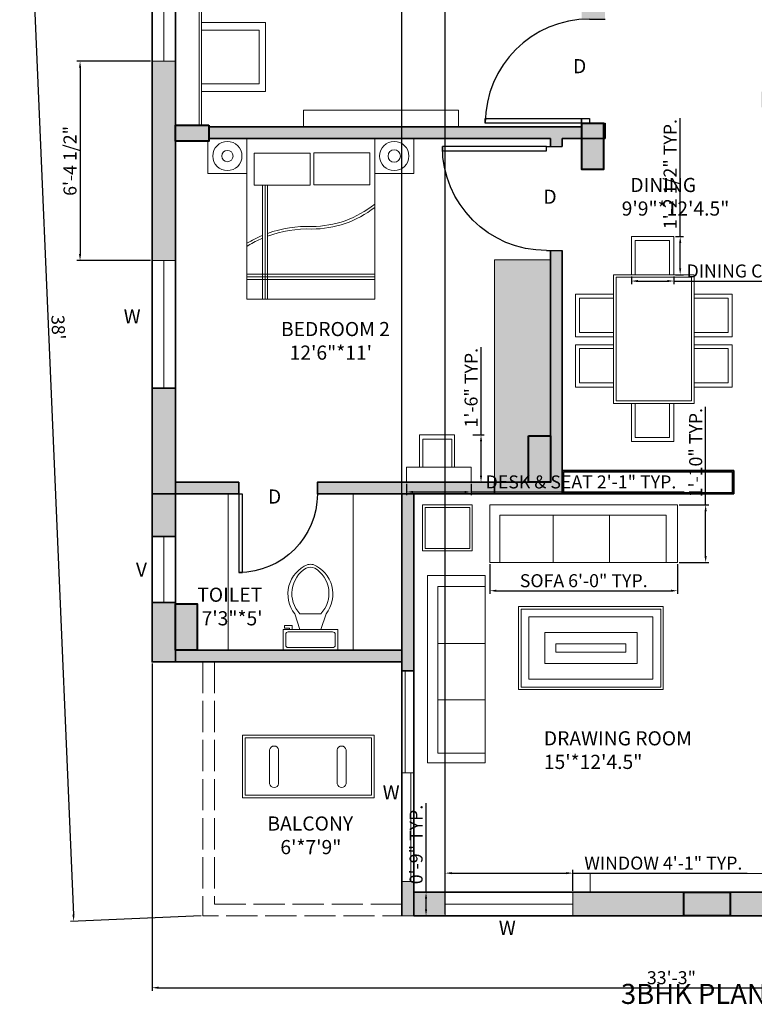
# Model space of a CAD drawing. Units: inches. Extents: x 351 to 1945, y 4338 to 4989.
# Tile 1 of 4: x 351 to 633, y 4338 to 4716. Entities that reach past the tile are written whole.
import ezdxf

# ---------------------------------------------------------------- set-up
doc = ezdxf.new("R2010")
doc.units = ezdxf.units.IN
doc.linetypes.add('ACAD_ISO02W100', pattern=[15, 12, -3])
for name, color, linetype, lineweight in [('A-ANNO-DIMS', 55, 'Continuous', 18), ('A-ANNO-IDEN', 55, 'Continuous', 18), ('A-ANNO-TEXT', 55, 'Continuous', 25), ('A-AREA-IDEN', 55, 'Continuous', 18), ('A-COLS-PATT', 210, 'Continuous', 13), ('A-FLOR-CASE', 30, 'Continuous', 20), ('A-FLOR-CASE-PATT', 30, 'Continuous', 13), ('A-FLOR-FIXT', 9, 'Continuous', 18), ('A-FLOR-RAIL', 7, 'ACAD_ISO02W100', 18), ('A-WALL-PATT', 130, 'Continuous', 13), ('COLUMN', 210, 'Continuous', 40), ('DOOR', 52, 'Continuous', 25), ('FUR', 142, 'Continuous', 18), ('WALL', 130, 'Continuous', 35), ('WIND', 10, 'Continuous', 20)]:
    doc.layers.add(name, color=color, linetype=linetype, lineweight=lineweight)
doc.styles.get("Standard").update_dxf_attribs({"font": 'arial.ttf'})
doc.dimstyles.new('ISO-25', dxfattribs={"dimtxt": 5, "dimasz": 2.5, "dimexe": 1.25, "dimexo": 0.625, "dimtad": 1, "dimdec": 0, "dimlunit": 4, "dimtxsty": 'Standard', "dimcen": 2.5, "dimadec": 0, "dimazin": 0, "dimtfac": 1, "dimtdec": 0, "dimtmove": 0, "dimatfit": 3, "dimfxl": 1, "dimarcsym": 0})

# ---------------------------------------------------------------- blocks, each defined once
blk = doc.blocks.new('*U2')
for p, q in [((0, 0), (0, -6)), ((40, 0), (40, -6))]:
    blk.add_line(p, q)
blk.add_lwpolyline([(0, 0), (0, 40), (1.75, 40), (1.75, 0)], close=True)
blk.add_arc((0, 0), 40, 0, 90)
blk = doc.blocks.new('*U4')
for p, q in [((9.5, -6), (9.5, -2)), ((-10, -8.5), (-8, -8.5)), ((-10, -9.5), (-10, -8.5)), ((-7, -9.5), (-10, -9.5)), ((-8, -8.5), (-8, -8)), ((-7, -8), (-7, -9.5)), ((-4, -8), (-6, -14)), ((4, -8), (6, -14)), ((4, -14), (-4, -14))]:
    blk.add_line(p, q)
blk.add_lwpolyline([(10.5, -8), (10.5, 0), (-10.5, 0), (-10.5, -8)], close=True)
for points in [[(-9.5, -2), (-9.5, -6)], [(8.5, -1), (-8.5, -1)], [(-8.5, -7), (8.5, -7)]]:
    blk.add_lwpolyline(points)
for centre, radius, start, end in [((-8.62, -1.88), 0.884, 81.8699, 188.1301), ((8.62, -1.88), 0.884, 351.8699, 98.1301), ((-8.62, -6.12), 0.884, 171.8699, 278.1301), ((8.62, -6.12), 0.884, 261.8699, 8.1301), ((3.52, -21.58), 12.17, 141.4691, 247.9714), ((4.2, -21.82), 11.33, 136.3677, 238.9468), ((-3.52, -21.58), 12.17, 292.0284, 38.5307), ((-4.2, -21.82), 11.33, 301.053, 43.6321), ((0, -27.88), 4, 245.7318, 294.2682), ((0, -29), 4, 254.8605, 285.1395)]:
    blk.add_arc(centre, radius, start, end)
blk = doc.blocks.new('*D6')
at = {"layer": 'A-ANNO-DIMS', "color": 0, "lineweight": -2, "transparency": 16777216}
for p, q in [((401.46, 4828.13), (351.25, 4825.99)), ((352.6, 4823.54), (371.89, 4372.54)), ((420.96, 4372.13), (370.75, 4369.99))]:
    blk.add_line(p, q, dxfattribs=at)
at = {"layer": 'A-ANNO-DIMS', "color": 0, "lineweight": 100, "transparency": 16777216}
for points in [[(353.02, 4823.56), (352.19, 4823.52), (352.5, 4826.04)], [(372.31, 4372.55), (371.48, 4372.52), (372, 4370.04)]]:
    blk.add_solid(points, dxfattribs=at)
at = {"layer": 'Defpoints', "color": 0, "lineweight": 100, "transparency": 16777216}
for p in [(402.08, 4828.16), (372, 4370.04), (421.58, 4372.16)]:
    blk.add_point(p, dxfattribs=at)
at = {"layer": 'A-ANNO-DIMS', "color": 0, "transparency": 16777216, "insert": (365.42, 4598.17), "char_height": 5, "attachment_point": 5, "rotation": 272.4487}
blk.add_mtext("38'", dxfattribs=at)
blk = doc.blocks.new('BED-DOUBLE')
for p, q in [((5.95, 43.76), (5.95, 0)), ((6.95, 43.76), (6.95, 0)), ((7.95, 43.76), (7.95, 0)), ((0.52, 20.56), (0, 20.22)), ((0, 9.54), (49.08, 9.54)), ((0, 8.54), (49.08, 8.54)), ((0, 7.54), (49.08, 7.54))]:
    blk.add_line(p, q)
for points in [[(0, 61.61), (49.08, 61.61), (49.08, 0), (0, 0)], [(2.84, 55.99), (24.35, 55.99), (24.35, 43.76), (2.84, 43.76)], [(25.67, 56.16), (47.18, 56.16), (47.18, 43.92), (25.67, 43.92)]]:
    blk.add_lwpolyline(points, close=True)
for centre, radius, start, end in [((24.92, 66.13), 38.24, 270, 309.1724), ((24.92, 66.13), 39.24, 270, 307.9925), ((23.4, -17.42), 45.34, 88.0757, 109.9277), ((23.4, -17.42), 44.34, 88.0757, 110.3969), ((23.4, -17.42), 45.34, 112.6404, 121.0693), ((23.4, -17.42), 44.34, 113.1804, 121.0693)]:
    blk.add_arc(centre, radius, start, end)
blk = doc.blocks.new('NIGHTSTAND-R')
blk.add_lwpolyline([(0, 13.33), (15.02, 13.33), (15.02, 0), (0, 0)], close=True)
for radius in [5.61, 2.37]:
    blk.add_circle((7.51, 6.66), radius)
blk = doc.blocks.new('SOFA-3SEAT')
for p, q in [((0, 0), (0, 22.17)), ((0, 22.17), (72.05, 22.17)), ((72.05, 0), (72.05, 22.17)), ((24.28, 0), (24.28, 18.21)), ((45.88, 0), (45.88, 18.21)), ((3.78, 0), (0, 0)), ((67.76, 0), (72.05, 0))]:
    blk.add_line(p, q)
blk.add_lwpolyline([(3.78, 18.21), (67.76, 18.21), (67.76, 0), (3.78, 0)], close=True)
blk = doc.blocks.new('CHAIR-DINING')
for p, q in [((0, 0), (0, 14.68)), ((0, 14.68), (16.27, 14.68)), ((16.27, 0), (16.27, 14.68))]:
    blk.add_line(p, q)
blk.add_lwpolyline([(1.45, 0), (14.67, 0), (14.67, 13.09), (1.45, 13.09)], close=True)
blk = doc.blocks.new('BEDROOM-DESK-AND-SEAT')
for p, q in [((5, 5.84), (5, 18.2)), ((5, 18.2), (18.5, 18.2)), ((18.5, 18.2), (18.5, 5.84))]:
    blk.add_line(p, q)
for points in [[(6.28, 5.84), (17.4, 5.84), (17.4, 16.62), (6.28, 16.62)], [(0, 0), (24.89, 0), (24.89, 5.84), (0, 5.84)]]:
    blk.add_lwpolyline(points, close=True)
blk = doc.blocks.new('WIN-49')
blk.add_line((0, 4.5), (49.03, 4.5))
blk.add_lwpolyline([(0, 0), (49.03, 0), (49.03, 9), (0, 9)], close=True)
blk = doc.blocks.new('*D15')
at = {"layer": 'A-ANNO-DIMS', "color": 0, "lineweight": -2, "transparency": 16777216}
for p, q in [((586.22, 4617.77), (586.22, 4614.71)), ((588.72, 4615.96), (599.99, 4615.96)), ((602.49, 4617.77), (602.49, 4614.71)), ((602.49, 4615.96), (698.18, 4615.96))]:
    blk.add_line(p, q, dxfattribs=at)
at = {"layer": 'A-ANNO-DIMS', "color": 0, "lineweight": 100, "transparency": 16777216}
for points in [[(588.72, 4616.38), (588.72, 4615.54), (586.22, 4615.96)], [(599.99, 4616.38), (599.99, 4615.54), (602.49, 4615.96)]]:
    blk.add_solid(points, dxfattribs=at)
at = {"layer": 'Defpoints', "color": 0, "lineweight": 100, "transparency": 16777216}
for p in [(586.22, 4618.4), (602.49, 4618.4), (602.49, 4615.96)]:
    blk.add_point(p, dxfattribs=at)
at = {"layer": 'A-ANNO-DIMS', "color": 0, "transparency": 16777216, "insert": (651.59, 4619.17), "char_height": 5, "attachment_point": 5}
blk.add_mtext('DINING CHAIR 1\'-4 1/2" TYP.', dxfattribs=at)
blk = doc.blocks.new('*D16')
at = {"layer": 'A-ANNO-DIMS', "color": 0, "lineweight": -2, "transparency": 16777216}
for p, q in [((604.93, 4633.08), (604.93, 4678.49)), ((603.12, 4633.08), (606.18, 4633.08)), ((604.93, 4620.9), (604.93, 4630.58)), ((603.12, 4618.4), (606.18, 4618.4))]:
    blk.add_line(p, q, dxfattribs=at)
at = {"layer": 'A-ANNO-DIMS', "color": 0, "lineweight": 100, "transparency": 16777216}
for points in [[(604.52, 4630.58), (605.35, 4630.58), (604.93, 4633.08)], [(604.52, 4620.9), (605.35, 4620.9), (604.93, 4618.4)]]:
    blk.add_solid(points, dxfattribs=at)
at = {"layer": 'Defpoints', "color": 0, "lineweight": 100, "transparency": 16777216}
for p in [(602.49, 4633.08), (604.93, 4633.08), (602.49, 4618.4)]:
    blk.add_point(p, dxfattribs=at)
at = {"layer": 'A-ANNO-DIMS', "color": 0, "transparency": 16777216, "insert": (601.72, 4657.04), "char_height": 5, "attachment_point": 5, "rotation": 90}
blk.add_mtext('1\'-2 1/2" TYP.', dxfattribs=at)
blk = doc.blocks.new('*D17')
at = {"layer": 'A-ANNO-DIMS', "color": 0, "lineweight": -2, "transparency": 16777216}
for p, q in [((514.67, 4381.78), (514.67, 4389.76)), ((517.17, 4388.51), (561.2, 4388.51)), ((563.7, 4381.78), (563.7, 4389.76)), ((563.7, 4388.51), (630.72, 4388.51))]:
    blk.add_line(p, q, dxfattribs=at)
at = {"layer": 'A-ANNO-DIMS', "color": 0, "lineweight": 100, "transparency": 16777216}
for points in [[(517.17, 4388.93), (517.17, 4388.1), (514.67, 4388.51)], [(561.2, 4388.93), (561.2, 4388.1), (563.7, 4388.51)]]:
    blk.add_solid(points, dxfattribs=at)
at = {"layer": 'Defpoints', "color": 0, "lineweight": 100, "transparency": 16777216}
for p in [(563.7, 4388.51), (514.67, 4381.16), (563.7, 4381.16)]:
    blk.add_point(p, dxfattribs=at)
at = {"layer": 'A-ANNO-DIMS', "color": 0, "transparency": 16777216, "insert": (598.46, 4391.73), "char_height": 5, "attachment_point": 5}
blk.add_mtext('WINDOW 4\'-1" TYP.', dxfattribs=at)
blk = doc.blocks.new('*D18')
at = {"layer": 'A-ANNO-DIMS', "color": 0, "lineweight": -2, "transparency": 16777216}
for p, q in [((507.32, 4381.16), (507.32, 4415.39)), ((514.05, 4381.16), (506.07, 4381.16)), ((507.32, 4374.66), (507.32, 4378.66)), ((514.05, 4372.16), (506.07, 4372.16))]:
    blk.add_line(p, q, dxfattribs=at)
at = {"layer": 'A-ANNO-DIMS', "color": 0, "lineweight": 100, "transparency": 16777216}
for points in [[(506.9, 4378.66), (507.74, 4378.66), (507.32, 4381.16)], [(506.9, 4374.66), (507.74, 4374.66), (507.32, 4372.16)]]:
    blk.add_solid(points, dxfattribs=at)
at = {"layer": 'Defpoints', "color": 0, "lineweight": 100, "transparency": 16777216}
for p in [(507.32, 4381.16), (514.67, 4381.16), (514.67, 4372.16)]:
    blk.add_point(p, dxfattribs=at)
at = {"layer": 'A-ANNO-DIMS', "color": 0, "transparency": 16777216, "insert": (504.14, 4399.52), "char_height": 5, "attachment_point": 5, "rotation": 90}
blk.add_mtext('0\'-9" TYP.', dxfattribs=at)
blk = doc.blocks.new('*D27')
at = {"layer": 'A-ANNO-DIMS', "color": 0, "lineweight": -2, "transparency": 16777216}
for p, q in [((531.85, 4507.18), (531.85, 4495.75)), ((603.9, 4507.18), (603.9, 4495.75)), ((534.35, 4497), (601.4, 4497))]:
    blk.add_line(p, q, dxfattribs=at)
at = {"layer": 'A-ANNO-DIMS', "color": 0, "lineweight": 100, "transparency": 16777216}
for points in [[(534.35, 4497.41), (534.35, 4496.58), (531.85, 4497)], [(601.4, 4497.41), (601.4, 4496.58), (603.9, 4497)]]:
    blk.add_solid(points, dxfattribs=at)
at = {"layer": 'Defpoints', "color": 0, "lineweight": 100, "transparency": 16777216}
for p in [(531.85, 4507.8), (603.9, 4507.8), (603.9, 4497)]:
    blk.add_point(p, dxfattribs=at)
at = {"layer": 'A-ANNO-DIMS', "color": 0, "transparency": 16777216, "insert": (567.88, 4500.21), "char_height": 5, "attachment_point": 5}
blk.add_mtext('SOFA 6\'-0" TYP.', dxfattribs=at)
blk = doc.blocks.new('*D28')
at = {"layer": 'A-ANNO-DIMS', "color": 0, "lineweight": -2, "transparency": 16777216}
for p, q in [((614.71, 4529.97), (614.71, 4567.61)), ((604.53, 4529.97), (615.96, 4529.97)), ((614.71, 4510.3), (614.71, 4527.47)), ((604.53, 4507.8), (615.96, 4507.8))]:
    blk.add_line(p, q, dxfattribs=at)
at = {"layer": 'A-ANNO-DIMS', "color": 0, "lineweight": 100, "transparency": 16777216}
for points in [[(614.29, 4527.47), (615.13, 4527.47), (614.71, 4529.97)], [(614.29, 4510.3), (615.13, 4510.3), (614.71, 4507.8)]]:
    blk.add_solid(points, dxfattribs=at)
at = {"layer": 'Defpoints', "color": 0, "lineweight": 100, "transparency": 16777216}
for p in [(603.9, 4529.97), (614.71, 4529.97), (603.9, 4507.8)]:
    blk.add_point(p, dxfattribs=at)
at = {"layer": 'A-ANNO-DIMS', "color": 0, "transparency": 16777216, "insert": (611.53, 4550.04), "char_height": 5, "attachment_point": 5, "rotation": 90}
blk.add_mtext('1\'-10" TYP.', dxfattribs=at)
blk = doc.blocks.new('*D29')
at = {"layer": 'A-ANNO-DIMS', "color": 0, "lineweight": -2, "transparency": 16777216}
for p, q in [((499.81, 4538.03), (499.81, 4533.68)), ((502.31, 4534.93), (522.21, 4534.93)), ((524.71, 4538.03), (524.71, 4533.68)), ((524.71, 4534.93), (606.43, 4534.93))]:
    blk.add_line(p, q, dxfattribs=at)
at = {"layer": 'A-ANNO-DIMS', "color": 0, "lineweight": 100, "transparency": 16777216}
for points in [[(502.31, 4535.34), (502.31, 4534.51), (499.81, 4534.93)], [(522.21, 4535.34), (522.21, 4534.51), (524.71, 4534.93)]]:
    blk.add_solid(points, dxfattribs=at)
at = {"layer": 'Defpoints', "color": 0, "lineweight": 100, "transparency": 16777216}
for p in [(499.81, 4538.66), (524.71, 4538.66), (524.71, 4534.93)]:
    blk.add_point(p, dxfattribs=at)
at = {"layer": 'A-ANNO-DIMS', "color": 0, "transparency": 16777216, "insert": (566.82, 4538.15), "char_height": 5, "attachment_point": 5}
blk.add_mtext('DESK & SEAT 2\'-1" TYP.', dxfattribs=at)
blk = doc.blocks.new('*D30')
at = {"layer": 'A-ANNO-DIMS', "color": 0, "lineweight": -2, "transparency": 16777216}
for p, q in [((528.44, 4556.86), (528.44, 4590.62)), ((525.33, 4556.86), (529.69, 4556.86)), ((528.44, 4541.16), (528.44, 4554.36)), ((525.33, 4538.66), (529.69, 4538.66))]:
    blk.add_line(p, q, dxfattribs=at)
at = {"layer": 'A-ANNO-DIMS', "color": 0, "lineweight": 100, "transparency": 16777216}
for points in [[(528.03, 4554.36), (528.86, 4554.36), (528.44, 4556.86)], [(528.03, 4541.16), (528.86, 4541.16), (528.44, 4538.66)]]:
    blk.add_solid(points, dxfattribs=at)
at = {"layer": 'Defpoints', "color": 0, "lineweight": 100, "transparency": 16777216}
for p in [(524.71, 4556.86), (528.44, 4556.86), (524.71, 4538.66)]:
    blk.add_point(p, dxfattribs=at)
at = {"layer": 'A-ANNO-DIMS', "color": 0, "transparency": 16777216, "insert": (525.27, 4574.99), "char_height": 5, "attachment_point": 5, "rotation": 90}
blk.add_mtext('1\'-6" TYP.', dxfattribs=at)
blk = doc.blocks.new('*D31')
at = {"layer": 'A-ANNO-DIMS', "color": 0, "lineweight": -2, "transparency": 16777216}
for p, q in [((402.08, 4469.03), (402.08, 4343.26)), ((801.08, 4371.53), (801.08, 4343.26)), ((404.58, 4344.51), (798.58, 4344.51))]:
    blk.add_line(p, q, dxfattribs=at)
at = {"layer": 'A-ANNO-DIMS', "color": 0, "lineweight": 100, "transparency": 16777216}
for points in [[(404.58, 4344.93), (404.58, 4344.09), (402.08, 4344.51)], [(798.58, 4344.93), (798.58, 4344.09), (801.08, 4344.51)]]:
    blk.add_solid(points, dxfattribs=at)
at = {"layer": 'Defpoints', "color": 0, "lineweight": 100, "transparency": 16777216}
for p in [(402.08, 4469.66), (801.08, 4372.16), (801.08, 4344.51)]:
    blk.add_point(p, dxfattribs=at)
at = {"layer": 'A-ANNO-DIMS', "color": 0, "transparency": 16777216, "insert": (601.58, 4347.69), "char_height": 5, "attachment_point": 5}
blk.add_mtext('33\'-3"', dxfattribs=at)
blk = doc.blocks.new('*D36')
at = {"layer": 'A-ANNO-DIMS', "color": 0, "lineweight": -2, "transparency": 16777216}
for p, q in [((401.46, 4700.38), (373.18, 4700.38)), ((374.43, 4697.88), (374.43, 4626.33)), ((401.46, 4623.83), (373.18, 4623.83))]:
    blk.add_line(p, q, dxfattribs=at)
at = {"layer": 'A-ANNO-DIMS', "color": 0, "lineweight": 100, "transparency": 16777216}
for points in [[(374.02, 4697.88), (374.85, 4697.88), (374.43, 4700.38)], [(374.02, 4626.33), (374.85, 4626.33), (374.43, 4623.83)]]:
    blk.add_solid(points, dxfattribs=at)
at = {"layer": 'Defpoints', "color": 0, "lineweight": 100, "transparency": 16777216}
for p in [(402.08, 4700.38), (374.43, 4623.83), (402.08, 4623.83)]:
    blk.add_point(p, dxfattribs=at)
at = {"layer": 'A-ANNO-DIMS', "color": 0, "transparency": 16777216, "insert": (371.22, 4662.11), "char_height": 5, "attachment_point": 5, "rotation": 90}
blk.add_mtext('6\'-4 1/2"', dxfattribs=at)
blk = doc.blocks.new('*D39')
at = {"layer": 'A-ANNO-DIMS', "color": 0, "lineweight": -2, "transparency": 16777216}
for p, q in [((498.08, 4372.78), (498.08, 4857.06)), ((514.67, 4372.78), (514.67, 4857.06)), ((500.58, 4855.81), (512.17, 4855.81)), ((514.67, 4855.81), (542.89, 4855.81))]:
    blk.add_line(p, q, dxfattribs=at)
at = {"layer": 'A-ANNO-DIMS', "color": 0, "lineweight": 100, "transparency": 16777216}
for points in [[(500.58, 4856.23), (500.58, 4855.39), (498.08, 4855.81)], [(512.17, 4856.23), (512.17, 4855.39), (514.67, 4855.81)]]:
    blk.add_solid(points, dxfattribs=at)
at = {"layer": 'Defpoints', "color": 0, "lineweight": 100, "transparency": 16777216}
for p in [(514.67, 4855.81), (498.08, 4372.16), (514.67, 4372.16)]:
    blk.add_point(p, dxfattribs=at)
at = {"layer": 'A-ANNO-DIMS', "color": 0, "transparency": 16777216, "insert": (530.03, 4859.02), "char_height": 5, "attachment_point": 5}
blk.add_mtext('1\'-4 1/2"', dxfattribs=at)

msp = doc.modelspace()

# ---------------------------------------------------------------- hatches: boundary and pattern name
at = {"layer": 'A-COLS-PATT'}
h = msp.add_hatch(color=256, dxfattribs=at)
h.dxf.hatch_style = 1
h.paths.add_polyline_path([(419.45, 4819.16), (411.08, 4819.16), (411.08, 4801.31), (419.45, 4801.31)])
h.paths.add_polyline_path([(760.58, 4819.16), (752.22, 4819.16), (752.22, 4801.31), (760.58, 4801.31)])
h.paths.add_polyline_path([(567.08, 4819.16), (558.72, 4819.16), (558.72, 4801.31), (567.08, 4801.31)])
h.paths.add_polyline_path([(423.85, 4675.88), (411.08, 4675.88), (411.08, 4669.65), (423.85, 4669.65)])
h.paths.add_polyline_path([(575.47, 4670.66), (567.1, 4670.66), (567.1, 4658.77), (575.47, 4658.77)])
h.paths.add_polyline_path([(575.47, 4676.62), (570.08, 4676.62), (567.1, 4676.62), (567.1, 4670.66), (575.47, 4670.66)])
h.paths.add_polyline_path([(769.58, 4687.16), (751.73, 4687.16), (751.73, 4682.66), (769.58, 4682.66)])
h.paths.add_polyline_path([(769.58, 4682.66), (751.73, 4682.66), (751.73, 4678.79), (769.58, 4678.79)])
h.paths.add_polyline_path([(514.67, 4381.16), (502.58, 4381.16), (502.58, 4372.16), (514.67, 4372.16)])
h.paths.add_polyline_path([(624.15, 4381.16), (606.3, 4381.16), (606.3, 4372.16), (624.15, 4372.16)])
h.paths.add_polyline_path([(752.08, 4381.16), (734.23, 4381.16), (734.23, 4372.16), (752.08, 4372.16)])
h.paths.add_polyline_path([(684.94, 4526.8), (676.58, 4526.8), (676.58, 4508.95), (684.94, 4508.95)])
h.paths.add_polyline_path([(419.45, 4492.01), (411.08, 4492.01), (411.08, 4474.16), (419.45, 4474.16)])
h.paths.add_polyline_path([(414.54, 4480.61), (443.82, 4480.61), (443.82, 4500.88), (414.54, 4500.88)], flags=9)
h = msp.add_hatch(color=256, dxfattribs=at)
h.dxf.hatch_style = 1
h.paths.add_polyline_path([(555.08, 4556.51), (546.72, 4556.51), (546.72, 4538.66), (555.08, 4538.66)])
h = msp.add_hatch(color=256, dxfattribs=at)
h.dxf.hatch_style = 1
h.paths.add_polyline_path([(419.45, 4492.01), (411.08, 4492.01), (411.08, 4474.16), (419.45, 4474.16)])
h = msp.add_hatch(color=256, dxfattribs=at)
h.dxf.hatch_style = 1
h.paths.add_polyline_path([(502.58, 4385.32), (498.08, 4385.32), (498.08, 4376.66), (498.08, 4372.16), (502.58, 4372.16)])
at = {"layer": 'A-FLOR-CASE-PATT'}
h = msp.add_hatch(color=256, dxfattribs=at)
h.dxf.hatch_style = 1
h.paths.add_polyline_path([(440.18, 4819.16), (419.45, 4819.16), (419.45, 4801.31), (411.08, 4801.31), (411.08, 4729.12), (440.18, 4729.12)])
h.paths.add_polyline_path([(760.58, 4704.97), (709.51, 4704.97), (709.51, 4687.16), (760.58, 4687.16)])
h.paths.add_polyline_path([(555.08, 4624.13), (533.62, 4624.13), (533.62, 4538.66), (546.72, 4538.66), (546.72, 4556.51), (555.08, 4556.51)])
at = {"layer": 'A-WALL-PATT'}
h = msp.add_hatch(color=256, dxfattribs=at)
h.dxf.hatch_style = 1
h.paths.add_polyline_path([(519.58, 4828.16), (519.58, 4819.16), (534.65, 4819.16), (567.08, 4819.16), (567.08, 4801.31), (567.08, 4783.74), (571.99, 4783.74), (576.08, 4783.74), (576.08, 4819.16), (636.08, 4819.16), (636.08, 4728.72), (640.58, 4728.72), (640.58, 4819.16), (684.63, 4819.16), (684.63, 4828.16), (640.58, 4828.16), (576.08, 4828.16)])
h.paths.add_polyline_path([(402.08, 4828.16), (402.08, 4749.41), (411.08, 4749.41), (411.08, 4819.16), (419.45, 4819.16), (470.55, 4819.16), (470.55, 4828.16)])
h.paths.add_polyline_path([(733.65, 4828.16), (733.65, 4819.16), (746.53, 4819.16), (760.58, 4819.16), (760.58, 4801.31), (760.58, 4765.23), (769.58, 4765.23), (769.58, 4828.16)])
h.paths.add_polyline_path([(402.08, 4670.66), (402.08, 4623.83), (411.08, 4623.83), (411.08, 4670.66), (411.08, 4675.88), (411.08, 4700.38), (402.08, 4700.38)])
h.paths.add_polyline_path([(555.08, 4670.66), (555.08, 4667.68), (559.58, 4667.68), (559.58, 4670.66), (567.1, 4670.66), (567.1, 4675.16), (423.95, 4675.16), (423.85, 4675.16), (423.85, 4670.66)])
h.paths.add_polyline_path([(576.08, 4727.66), (576.08, 4751.3, -0.031413), (571.99, 4751.04), (567.08, 4751.04), (567.08, 4716.51, -0.01877), (570.08, 4716.62), (576.08, 4716.62), (576.08, 4723.16), (636.08, 4723.16), (640.58, 4723.16), (640.58, 4728.72), (636.08, 4728.72), (636.08, 4727.66)])
h.paths.add_polyline_path([(672.08, 4682.66), (672.08, 4641.87), (676.58, 4641.87), (676.58, 4682.66), (724.58, 4682.66), (724.58, 4677.41), (729.08, 4677.41), (729.08, 4682.66), (751.73, 4682.66), (751.73, 4687.16), (709.51, 4687.16), (684.61, 4687.16), (640.58, 4687.16), (640.58, 4688.72), (636.08, 4688.72), (636.08, 4682.66)])
h.paths.add_polyline_path([(753.8, 4463.91), (782.66, 4463.91), (782.66, 4484.16), (753.8, 4484.16)], flags=9)
h.paths.add_polyline_path([(760.86, 4391.5), (776.24, 4391.5), (776.24, 4411.77), (760.86, 4411.77)], flags=9)
h.paths.add_polyline_path([(690.04, 4455.43), (720.56, 4455.43), (720.56, 4475.7), (690.04, 4475.7)], flags=9)
h.paths.add_polyline_path([(676.19, 4400.06), (720.94, 4400.06), (720.94, 4420.3), (676.19, 4420.3)], flags=9)
h.paths.add_polyline_path([(550.38, 4425.45), (615.73, 4425.45), (615.73, 4445.72), (550.38, 4445.72)], flags=9)
h.paths.add_polyline_path([(417.92, 4480.61), (447.2, 4480.61), (447.2, 4500.88), (417.92, 4500.88)], flags=9)
h.paths.add_polyline_path([(449.69, 4582.66), (497.94, 4582.66), (497.94, 4602.93), (449.69, 4602.93)], flags=9)
h.paths.add_polyline_path([(580.8, 4638.02), (622.18, 4638.02), (622.18, 4658.29), (580.8, 4658.29)], flags=9)
h.paths.add_polyline_path([(748.64, 4653.12), (792.13, 4653.12), (792.13, 4673.39), (748.64, 4673.39)], flags=9)
h.paths.add_polyline_path([(686.44, 4648.7), (715.72, 4648.7), (715.72, 4668.97), (686.44, 4668.97)], flags=25)
h.paths.add_polyline_path([(689.64, 4550.87), (725.93, 4550.87), (725.93, 4571.14), (689.64, 4571.14)], flags=9)
h.paths.add_polyline_path([(671.27, 4732.55), (719.52, 4732.55), (719.52, 4752.82), (671.27, 4752.82)], flags=9)
h.paths.add_polyline_path([(458.57, 4731.55), (540.55, 4731.55), (540.55, 4751.82), (458.57, 4751.82)], flags=9)
h = msp.add_hatch(color=256, dxfattribs=at)
h.dxf.hatch_style = 1
h.paths.add_polyline_path([(729.08, 4663.38), (724.58, 4663.38), (724.58, 4610.66), (676.58, 4610.66), (676.58, 4612.12), (676.55, 4612.12), (672.08, 4612.12), (672.08, 4606.16), (672.08, 4581.14), (676.58, 4581.14), (676.58, 4606.16), (729.08, 4606.16), (730.91, 4606.16), (730.91, 4610.66), (729.08, 4610.66)])
h.paths.add_polyline_path([(676.58, 4507.65), (676.58, 4508.95), (676.58, 4508.95), (676.58, 4526.98), (672.08, 4526.98), (672.08, 4489.16), (676.58, 4489.16), (687.08, 4489.16), (747.58, 4489.16), (747.58, 4445.66), (742.58, 4445.66), (687.08, 4445.66), (676.58, 4445.66), (672.08, 4445.66), (672.08, 4424.71), (676.58, 4424.71), (676.58, 4441.16), (687.08, 4441.16), (747.08, 4441.16), (747.08, 4423.66), (752.08, 4423.66), (752.08, 4445.66), (752.08, 4458.62), (752.08, 4489.16), (752.08, 4493.66), (676.58, 4493.66)])
h.paths.add_polyline_path([(734.23, 4381.16), (687.08, 4381.16), (680.85, 4381.16), (624.15, 4381.16), (624.15, 4372.16), (687.08, 4372.16), (734.23, 4372.16)])
h.paths.add_polyline_path([(606.3, 4381.16), (570.36, 4381.16), (563.7, 4381.16), (563.7, 4372.16), (606.3, 4372.16)])
h.paths.add_polyline_path([(753.8, 4463.91), (782.66, 4463.91), (782.66, 4484.16), (753.8, 4484.16)], flags=9)
h.paths.add_polyline_path([(760.86, 4391.5), (776.24, 4391.5), (776.24, 4411.77), (760.86, 4411.77)], flags=9)
h.paths.add_polyline_path([(690.04, 4455.43), (720.56, 4455.43), (720.56, 4475.7), (690.04, 4475.7)], flags=25)
h.paths.add_polyline_path([(676.19, 4400.06), (720.94, 4400.06), (720.94, 4420.3), (676.19, 4420.3)], flags=9)
h.paths.add_polyline_path([(550.38, 4425.45), (615.73, 4425.45), (615.73, 4445.72), (550.38, 4445.72)], flags=9)
h.paths.add_polyline_path([(417.92, 4480.61), (447.2, 4480.61), (447.2, 4500.88), (417.92, 4500.88)], flags=9)
h.paths.add_polyline_path([(449.69, 4582.66), (497.94, 4582.66), (497.94, 4602.93), (449.69, 4602.93)], flags=9)
h.paths.add_polyline_path([(580.8, 4638.02), (622.18, 4638.02), (622.18, 4658.29), (580.8, 4658.29)], flags=9)
h.paths.add_polyline_path([(748.64, 4653.12), (792.13, 4653.12), (792.13, 4673.39), (748.64, 4673.39)], flags=9)
h.paths.add_polyline_path([(686.44, 4648.7), (715.72, 4648.7), (715.72, 4668.97), (686.44, 4668.97)], flags=9)
h.paths.add_polyline_path([(689.64, 4550.87), (725.93, 4550.87), (725.93, 4571.14), (689.64, 4571.14)], flags=9)
h.paths.add_polyline_path([(671.27, 4732.55), (719.52, 4732.55), (719.52, 4752.82), (671.27, 4752.82)], flags=9)
h.paths.add_polyline_path([(594.05, 4791.87), (624.3, 4791.87), (624.3, 4812.11), (594.05, 4812.11)], flags=9)
h.paths.add_polyline_path([(458.57, 4731.55), (540.55, 4731.55), (540.55, 4751.82), (458.57, 4751.82)], flags=9)
h = msp.add_hatch(color=256, dxfattribs=at)
h.dxf.hatch_style = 1
h.paths.add_polyline_path([(769.58, 4716.2), (760.66, 4716.2), (760.66, 4687.16), (769.58, 4687.16)])
h.paths.add_polyline_path([(801.08, 4687.16), (796.58, 4687.16), (796.58, 4436.66), (801.08, 4436.66)])
h.paths.add_polyline_path([(411.08, 4574.8), (402.08, 4574.8), (402.08, 4534.16), (411.08, 4534.16), (411.08, 4538.66)])
h.paths.add_polyline_path([(411.08, 4534.16), (402.08, 4534.16), (402.08, 4517.84), (411.08, 4517.84)])
h.paths.add_polyline_path([(435.45, 4538.66), (411.08, 4538.66), (411.08, 4534.16), (435.45, 4534.16)])
h.paths.add_polyline_path([(411.08, 4492.45), (402.08, 4492.45), (402.08, 4469.66), (411.08, 4469.66)])
h.paths.add_polyline_path([(498.08, 4474.16), (411.08, 4474.16), (411.08, 4469.66), (498.08, 4469.66)])
h.paths.add_polyline_path([(502.58, 4534.16), (498.08, 4534.16), (498.08, 4466.28), (502.58, 4466.28)])
h.paths.add_polyline_path([(533.62, 4538.66), (465.58, 4538.66), (465.58, 4534.16), (533.62, 4534.16)])
h.paths.add_polyline_path([(559.58, 4627.68), (555.08, 4627.68), (555.08, 4538.66), (546.72, 4538.66), (533.62, 4538.66), (533.62, 4534.16), (559.58, 4534.16)])

# ---------------------------------------------------------------- linework, layer by layer
at = {"layer": 'A-FLOR-CASE'}
for p, q in [((420.12, 4729.12), (420.12, 4675.88)), ((421.12, 4729.12), (421.12, 4675.88))]:
    msp.add_line(p, q, dxfattribs=at)
for points in [[(460.2, 4675.16), (519.85, 4675.16), (519.85, 4681.55), (460.2, 4681.55)], [(555.08, 4624.13), (533.62, 4624.13), (533.62, 4538.66), (555.08, 4538.66)], [(570.36, 4381.16), (642.24, 4381.16), (642.24, 4388.42), (570.36, 4388.42)]]:
    msp.add_lwpolyline(points, close=True, dxfattribs=at)
at = {"layer": 'A-FLOR-FIXT'}
for p, q in [((431.3, 4534.16), (431.3, 4474.16)), ((479.39, 4534.16), (479.39, 4474.16))]:
    msp.add_line(p, q, dxfattribs=at)
at = {"layer": 'A-FLOR-RAIL'}
for p, q in [((421.58, 4469.66), (421.58, 4372.16)), ((426.08, 4469.66), (426.08, 4376.66)), ((498.08, 4376.66), (426.08, 4376.66)), ((502.58, 4372.16), (421.58, 4372.16))]:
    msp.add_line(p, q, dxfattribs=at)
at = {"layer": 'COLUMN'}
for points in [[(423.85, 4675.88), (423.85, 4669.65), (411.08, 4669.65), (411.08, 4675.88)], [(567.1, 4676.62), (575.47, 4676.62), (575.47, 4658.77), (567.1, 4658.77)], [(546.72, 4556.51), (555.08, 4556.51), (555.08, 4538.66), (546.72, 4538.66)], [(411.08, 4492.01), (419.45, 4492.01), (419.45, 4474.16), (411.08, 4474.16)], [(624.15, 4381.16), (624.15, 4372.16), (606.3, 4372.16), (606.3, 4381.16)]]:
    msp.add_lwpolyline(points, close=True, dxfattribs=at)
at = {"layer": 'FUR'}
for p, q in [((445.72, 4715.32), (421.12, 4715.32)), ((445.72, 4688.76), (445.72, 4715.32)), ((421.12, 4688.76), (445.72, 4688.76))]:
    msp.add_line(p, q, dxfattribs=at)
for points in [[(421.12, 4691.77), (443.26, 4691.77), (443.26, 4712.38), (421.12, 4712.38)], [(579.35, 4568.95), (610.28, 4568.95), (610.28, 4618.4), (579.35, 4618.4)], [(580.35, 4569.95), (609.28, 4569.95), (609.28, 4617.4), (580.35, 4617.4)], [(505.93, 4529.97), (525.1, 4529.97), (525.1, 4512.28), (505.93, 4512.28)], [(506.93, 4528.97), (524.1, 4528.97), (524.1, 4513.28), (506.93, 4513.28)], [(542.83, 4490.98), (598.46, 4490.98), (598.46, 4459.01), (542.83, 4459.01)], [(543.83, 4489.98), (597.46, 4489.98), (597.46, 4460.01), (543.83, 4460.01)], [(546.83, 4486.98), (594.46, 4486.98), (594.46, 4463.01), (546.83, 4463.01)], [(552.9, 4480.91), (588.4, 4480.91), (588.4, 4469.08), (552.9, 4469.08)], [(557.22, 4476.59), (584.07, 4476.59), (584.07, 4473.4), (557.22, 4473.4)], [(436.84, 4441.48), (487.38, 4441.48), (487.38, 4417.42), (436.84, 4417.42)], [(437.84, 4440.48), (486.38, 4440.48), (486.38, 4418.42), (437.84, 4418.42)]]:
    msp.add_lwpolyline(points, close=True, dxfattribs=at)
for points in [[(423.87, 4670.66), (438.52, 4670.66), (438.52, 4657.33), (423.5, 4657.33), (423.5, 4669.65)], [(447.25, 4435.86), (447.25, 4422.87)], [(450.69, 4422.87), (450.69, 4435.86)], [(473.18, 4435.86), (473.18, 4422.87)], [(476.61, 4422.87), (476.61, 4435.86)]]:
    msp.add_lwpolyline(points, dxfattribs=at)
for radius in [5.61, 2.18]:
    msp.add_circle((431.01, 4663.99), radius, dxfattribs=at)
for centre, radius, start, end in [((448.97, 4435.61), 1.73, 7.996, 172.004), ((474.89, 4435.61), 1.73, 7.996, 172.004), ((448.97, 4423.2), 1.75, 191.0941, 348.9059), ((474.89, 4423.2), 1.75, 191.0941, 348.9059)]:
    msp.add_arc(centre, radius, start, end, dxfattribs=at)
at = {"layer": 'WALL'}
for p, q in [((402.08, 4670.66), (402.08, 4828.16)), ((411.08, 4675.16), (411.08, 4819.16)), ((411.18, 4675.16), (411.08, 4675.16)), ((423.95, 4675.16), (423.85, 4675.16)), ((567.08, 4675.16), (423.95, 4675.16)), ((567.08, 4678.37), (567.08, 4675.16)), ((576.08, 4676.62), (576.08, 4670.66)), ((402.08, 4670.66), (402.08, 4534.16)), ((411.08, 4670.66), (411.08, 4538.66)), ((411.08, 4670.66), (411.08, 4538.66)), ((411.1, 4670.66), (411.08, 4670.66)), ((555.08, 4670.66), (423.85, 4670.66)), ((555.08, 4667.68), (555.08, 4670.66)), ((576.08, 4670.66), (559.58, 4670.66)), ((559.58, 4670.66), (576.08, 4670.66)), ((559.58, 4667.68), (559.58, 4670.66)), ((555.08, 4538.66), (555.08, 4627.68)), ((559.58, 4534.16), (559.58, 4627.68)), ((625.53, 4543.16), (559.58, 4543.16)), ((625.03, 4542.66), (560.08, 4542.66)), ((560.08, 4534.66), (560.08, 4542.66)), ((625.03, 4534.66), (625.03, 4542.66)), ((625.53, 4534.16), (625.53, 4543.16)), ((411.08, 4538.66), (435.45, 4538.66)), ((411.08, 4538.66), (435.45, 4538.66)), ((465.58, 4538.66), (555.08, 4538.66)), ((465.58, 4538.66), (555.08, 4538.66)), ((502.58, 4538.66), (555.08, 4538.66)), ((402.08, 4534.16), (402.08, 4469.66)), ((411.08, 4534.16), (435.45, 4534.16)), ((411.08, 4534.16), (411.08, 4474.16)), ((465.58, 4534.16), (498.08, 4534.16)), ((498.08, 4474.16), (498.08, 4534.16)), ((502.58, 4469.66), (502.58, 4534.16)), ((502.58, 4534.16), (559.58, 4534.16)), ((502.58, 4534.16), (559.58, 4534.16)), ((559.58, 4534.16), (625.53, 4534.16)), ((560.08, 4534.66), (625.03, 4534.66)), ((502.58, 4381.16), (502.58, 4529.66)), ((411.08, 4474.16), (498.08, 4474.16)), ((402.08, 4469.66), (421.58, 4469.66)), ((426.08, 4469.66), (498.08, 4469.66)), ((498.08, 4469.66), (498.08, 4376.66)), ((502.58, 4469.66), (502.58, 4372.16)), ((502.58, 4381.16), (682.58, 4381.16)), ((498.08, 4376.66), (498.08, 4372.16)), ((502.58, 4372.16), (687.08, 4372.16))]:
    msp.add_line(p, q, dxfattribs=at)
for points in [[(402.08, 4574.8), (411.08, 4574.8), (411.08, 4534.16), (402.08, 4534.16)], [(435.45, 4538.66), (411.08, 4538.66), (411.08, 4534.16), (435.45, 4534.16)], [(465.58, 4534.16), (533.62, 4534.16), (533.62, 4538.66), (465.58, 4538.66)], [(402.08, 4517.84), (411.08, 4517.84), (411.08, 4534.16), (402.08, 4534.16)], [(498.08, 4534.16), (502.58, 4534.16), (502.58, 4466.28), (498.08, 4466.28)], [(402.08, 4492.45), (411.08, 4492.45), (411.08, 4469.66), (402.08, 4469.66)], [(498.08, 4469.66), (411.08, 4469.66), (411.08, 4474.16), (498.08, 4474.16)]]:
    msp.add_lwpolyline(points, close=True, dxfattribs=at)
at = {"layer": 'WIND'}
for p, q in [((406.58, 4492.45), (406.58, 4517.84)), ((498.08, 4466.28), (502.58, 4466.28)), ((498.08, 4385.32), (498.08, 4466.28)), ((499.32, 4466.28), (499.32, 4426.99)), ((502.58, 4385.32), (502.58, 4466.28)), ((502.58, 4426.99), (498.08, 4426.99)), ((501.42, 4426.99), (501.42, 4385.32)), ((498.08, 4385.32), (502.58, 4385.32))]:
    msp.add_line(p, q, dxfattribs=at)
msp.add_lwpolyline([(411.08, 4492.45), (402.08, 4492.45), (402.08, 4517.84), (411.08, 4517.84)], close=True, dxfattribs=at)

# ---------------------------------------------------------------- block references
at = {"layer": 'A-FLOR-FIXT', "xscale": -1, "rotation": 180}
msp.add_blockref('*U4', (462.91, 4474.16), dxfattribs=at)
at = {"layer": 'DOOR', "rotation": 90}
msp.add_blockref('*U2', (570.08, 4676.62), dxfattribs=at)
at = {"layer": 'DOOR', "xscale": -1, "rotation": 90}
msp.add_blockref('*U2', (553.58, 4667.68), dxfattribs=at)
at = {"layer": 'DOOR', "xscale": -0.753207244064139, "yscale": 0.753207244064139, "zscale": 0.753207244064139, "rotation": 180}
msp.add_blockref('*U2', (435.45, 4534.14), dxfattribs=at)
at = {"layer": 'FUR'}
for name, p in [('BED-DOUBLE', (438.52, 4609.05)), ('NIGHTSTAND-R', (487.6, 4657.33)), ('CHAIR-DINING', (586.22, 4618.4)), ('BEDROOM-DESK-AND-SEAT', (499.81, 4538.66)), ('SOFA-3SEAT', (531.85, 4507.8))]:
    msp.add_blockref(name, p, dxfattribs=at)
at = {"layer": 'FUR', "extrusion": (0, 0, -1), "zscale": -1}
for p, rotation in [((-579.35, 4610.86), 270.0000000000057), ((-579.35, 4591.5), 270.0000000000057), ((-586.22, 4568.95), 180)]:
    msp.add_blockref('CHAIR-DINING', p, dxfattribs=dict(at, rotation=rotation))
at = {"layer": 'FUR'}
for name, p, rotation in [('CHAIR-DINING', (610.28, 4610.86), 270.0000000000053), ('CHAIR-DINING', (610.28, 4591.5), 270.0000000000053), ('SOFA-3SEAT', (530.05, 4430.86), 89.99999999999898)]:
    msp.add_blockref(name, p, dxfattribs=dict(at, rotation=rotation))
at = {"layer": 'WIND', "rotation": 270.0000000000006}
for p in [(402.08, 4749.41), (402.08, 4623.83)]:
    msp.add_blockref('WIN-49', p, dxfattribs=at)
at = {"layer": 'WIND'}
msp.add_blockref('WIN-49', (514.67, 4372.16), dxfattribs=at)

# ---------------------------------------------------------------- texts
at = {"layer": 'A-ANNO-IDEN', "char_height": 5.43, "attachment_point": 1}
for s, insert in [('D', (563.78, 4701.22)), ('D', (552.4, 4651.07)), ('W', (391.19, 4605.12)), ('D', (446.6, 4535.89)), ('V', (395.88, 4507.84)), ('W', (490.67, 4422.26)), ('W', (535.27, 4370.23))]:
    msp.add_mtext_dynamic_manual_height_columns(s, width=132.0225, gutter_width=27.16, heights=[0], dxfattribs=dict(at, insert=insert))
at = {"layer": 'A-ANNO-TEXT', "insert": (582.18, 4345.99), "char_height": 7.723, "attachment_point": 1}
msp.add_mtext_dynamic_manual_height_columns('3BHK PLAN', width=489.8705, gutter_width=38.61, heights=[0], dxfattribs=at)
at = {"layer": 'A-AREA-IDEN', "attachment_point": 1}
for s, insert, char_height in [('  DINING\\P9\'9"*12\'4.5"', (582.47, 4655.58), 5.4321), ('BEDROOM 2\\P  12\'6"*11\'', (451.6, 4600.23), 5.4321), ('TOILET\\P 7\'3"*5\'', (419.45, 4498.18), 5.432), ('DRAWING ROOM\\P15\'*12\'4.5"', (552.57, 4443.02), 5.4321), ('BALCONY\\P   6\'*7\'9"', (446.39, 4410.29), 5.432)]:
    msp.add_mtext_dynamic_manual_height_columns(s, width=132.0225, gutter_width=27.16, heights=[0], dxfattribs=dict(at, insert=insert, char_height=char_height))

# ---------------------------------------------------------------- dimensions: what is measured, and where the dimension line sits
at = {"layer": 'A-ANNO-DIMS'}
for base, p1, p2, picture, middle in [((514.67, 4855.81), (498.08, 4372.16), (514.67, 4372.16), '*D39', (530.03, 4859.02)), ((801.08, 4344.51), (402.08, 4469.66), (801.08, 4372.16), '*D31', (601.58, 4347.69))]:
    dim = msp.add_linear_dim(base=base, p1=p1, p2=p2, dimstyle='ISO-25', override={"dimdec": 1, "dimlfac": 1, "dimrnd": 0, "dimzin": 1, "dimdsep": 46, "dimlunit": 4, "dimfrac": 2}, dxfattribs=at)
    dim.commit()
    dim.dimension.update_dxf_attribs({"geometry": picture, "text_midpoint": middle})
dim = msp.add_aligned_dim(p1=(402.08, 4828.16), p2=(421.58, 4372.16), distance=-49.63, dimstyle='ISO-25', override={"dimclrd": 0, "dimclre": 0, "dimclrt": 0}, dxfattribs=at)
dim.commit()
dim.dimension.update_dxf_attribs({"geometry": '*D6', "text_midpoint": (365.42, 4598.17)})
dim = msp.add_linear_dim(base=(374.4348, 4623.8322), p1=(402.0848, 4700.381), p2=(402.0848, 4623.8322), angle=90, dimstyle='ISO-25', override={"dimdec": 1, "dimlfac": 1, "dimrnd": 0, "dimzin": 1, "dimdsep": 46, "dimlunit": 4, "dimfrac": 2}, dxfattribs=at)
dim.commit()
dim.dimension.update_dxf_attribs({"geometry": '*D36', "text_midpoint": (371.2246, 4662.1066)})
for base, p1, p2, picture, middle in [((604.93, 4633.08), (602.49, 4618.4), (602.49, 4633.08), '*D16', (601.72, 4657.04)), ((528.44, 4556.86), (524.71, 4538.66), (524.71, 4556.86), '*D30', (525.27, 4574.99)), ((614.71, 4529.97), (603.9, 4507.8), (603.9, 4529.97), '*D28', (611.53, 4550.04)), ((507.32, 4381.16), (514.67, 4372.16), (514.67, 4381.16), '*D18', (504.14, 4399.52))]:
    dim = msp.add_linear_dim(base=base, p1=p1, p2=p2, angle=90, text='<> TYP.', dimstyle='ISO-25', override={"dimdec": 1, "dimlfac": 1, "dimrnd": 0, "dimzin": 1, "dimdsep": 46, "dimlunit": 4, "dimfrac": 2}, dxfattribs=at)
    dim.commit()
    dim.dimension.update_dxf_attribs({"geometry": picture, "text_midpoint": middle})
for base, p1, p2, text, picture, middle in [((602.49, 4615.96), (586.22, 4618.4), (602.49, 4618.4), 'DINING CHAIR <> TYP.', '*D15', (651.59, 4619.17)), ((524.71, 4534.93), (499.81, 4538.66), (524.71, 4538.66), 'DESK & SEAT <> TYP.', '*D29', (566.82, 4538.15)), ((603.9033, 4496.9963), (531.8487, 4507.8045), (603.9033, 4507.8045), 'SOFA <> TYP.', '*D27', (567.876, 4500.2083)), ((563.7, 4388.51), (514.67, 4381.16), (563.7, 4381.16), 'WINDOW <> TYP.', '*D17', (598.46, 4391.73))]:
    dim = msp.add_linear_dim(base=base, p1=p1, p2=p2, text=text, dimstyle='ISO-25', override={"dimdec": 1, "dimlfac": 1, "dimrnd": 0, "dimzin": 1, "dimdsep": 46, "dimlunit": 4, "dimfrac": 2}, dxfattribs=at)
    dim.commit()
    dim.dimension.update_dxf_attribs({"geometry": picture, "text_midpoint": middle})

doc.saveas('drawing.dxf')
